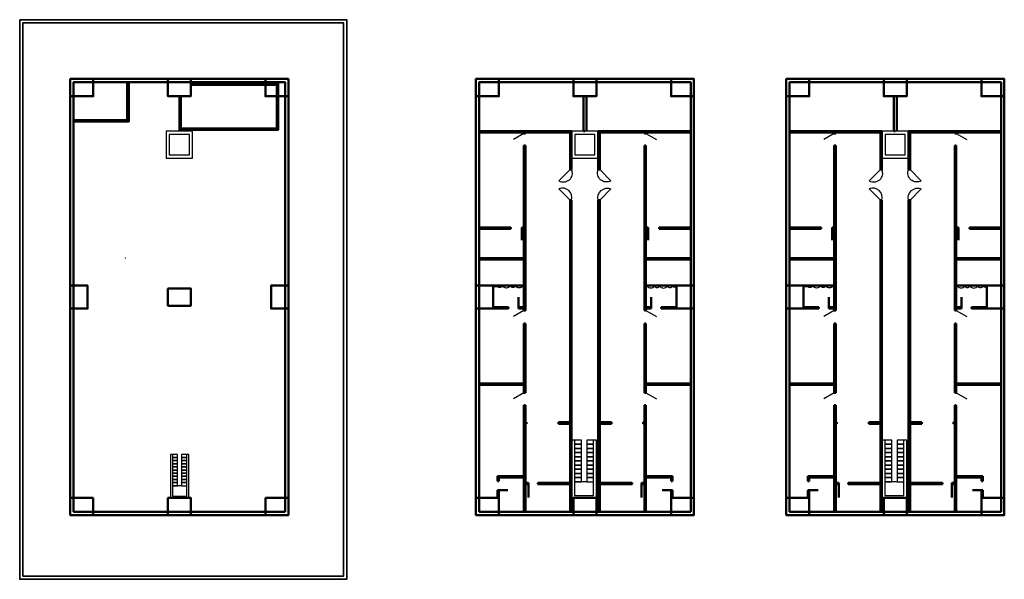
# Model space of a CAD drawing. Units: feet. Extents: x 1080 to 13444, y 870 to 7060.
# Tile 1 of 5: x 1080 to 3789, y 870 to 2410. Entities that reach past the tile are written whole.
import ezdxf

# ---------------------------------------------------------------- set-up
doc = ezdxf.new("R2010")
doc.units = ezdxf.units.FT
for name, color, linetype, lineweight in [('A-ANNO-NPLT', 8, 'Continuous', 13), ('A-COLS', 1, 'Continuous', 50), ('A-DOOR', 4, 'Continuous', 25), ('A-FLOR-EVTR', 6, 'Continuous', 25), ('A-FLOR-STRS', 2, 'Continuous', 25), ('A-GLAZ', 3, 'Continuous', 25), ('A-WALL', 7, 'Continuous', 50), ('C-PROP', 3, 'Continuous', 35)]:
    doc.layers.add(name, color=color, linetype=linetype, lineweight=lineweight)

# ---------------------------------------------------------------- blocks, each defined once
blk = doc.blocks.new('DOOR-SWING-A')
blk.add_line((30.9, 34), (0, 3.5))
blk.add_arc((12.6, 24.3), 24.3, 238.69, 23.7025)
blk = doc.blocks.new('DOOR-SWING-B')
blk.add_line((0, 30.5), (30.9, 0))
blk.add_arc((10.2, 7), 25.6, 344.0766, 113.531)

msp = doc.modelspace()

# ---------------------------------------------------------------- linework, layer by layer
at = {"layer": 'A-ANNO-NPLT'}
for p in [(1370.9, 1754.2), (2471.5, 1405), (2799.2, 1405), (3325.4, 1405), (3653.1, 1405)]:
    msp.add_point(p, dxfattribs=at)
at = {"layer": 'A-COLS'}
for points in [[(1219.3, 2246.8), (1282.3, 2246.8), (1282.3, 2199.1), (1219.3, 2199.1)], [(1487.8, 2246.8), (1550.8, 2246.8), (1550.8, 2199.1), (1487.8, 2199.1)], [(1756.3, 2246.8), (1819.3, 2246.8), (1819.3, 2199.1), (1756.3, 2199.1)], [(2335.3, 2246.8), (2398.4, 2246.8), (2398.4, 2199.1), (2335.3, 2199.1)], [(2603.8, 2246.8), (2666.8, 2246.8), (2666.8, 2199.1), (2603.8, 2199.1)], [(2872.3, 2246.8), (2935.3, 2246.8), (2935.3, 2199.1), (2872.3, 2199.1)], [(3189.2, 2246.8), (3252.3, 2246.8), (3252.3, 2199.1), (3189.2, 2199.1)], [(3457.7, 2246.8), (3520.7, 2246.8), (3520.7, 2199.1), (3457.7, 2199.1)], [(3726.2, 2246.8), (3789.2, 2246.8), (3789.2, 2199.1), (3726.2, 2199.1)], [(1219.3, 1615.2), (1219.3, 1678.3), (1266.9, 1678.3), (1266.9, 1615.2)], [(1487.8, 1670.6), (1550.8, 1670.6), (1550.8, 1622.9), (1487.8, 1622.9)], [(1819.3, 1678.3), (1819.3, 1615.2), (1771.6, 1615.2), (1771.6, 1678.3)], [(2335.3, 1615.2), (2335.3, 1678.3), (2383, 1678.3), (2383, 1615.2)], [(2935.3, 1678.3), (2935.3, 1615.2), (2887.7, 1615.2), (2887.7, 1678.3)], [(3189.2, 1615.2), (3189.2, 1678.3), (3236.9, 1678.3), (3236.9, 1615.2)], [(3789.2, 1678.3), (3789.2, 1615.2), (3741.6, 1615.2), (3741.6, 1678.3)], [(1282.3, 1094.4), (1219.3, 1094.4), (1219.3, 1046.8), (1282.3, 1046.8)], [(1487.8, 1094.4), (1550.8, 1094.4), (1550.8, 1046.8), (1487.8, 1046.8)], [(1756.3, 1094.4), (1819.3, 1094.4), (1819.3, 1046.8), (1756.3, 1046.8)], [(2398.4, 1094.4), (2335.3, 1094.4), (2335.3, 1046.8), (2398.4, 1046.8)], [(2666.8, 1046.8), (2603.8, 1046.8), (2603.8, 1094.4), (2666.8, 1094.4)], [(2872.3, 1094.4), (2935.3, 1094.4), (2935.3, 1046.8), (2872.3, 1046.8)], [(3252.3, 1094.4), (3189.2, 1094.4), (3189.2, 1046.8), (3252.3, 1046.8)], [(3520.7, 1046.8), (3457.7, 1046.8), (3457.7, 1094.4), (3520.7, 1094.4)], [(3726.2, 1094.4), (3789.2, 1094.4), (3789.2, 1046.8), (3726.2, 1046.8)]]:
    msp.add_lwpolyline(points, close=True, dxfattribs=at)
at = {"layer": 'A-DOOR'}
for p, q in [((2467.5, 2096.8), (2438.6, 2080.5)), ((2803.2, 2096.8), (2832.1, 2080.5)), ((3321.4, 2096.8), (3292.5, 2080.5)), ((3657.1, 2096.8), (3686, 2080.5)), ((2467.5, 1609.3), (2438.6, 1593)), ((2803.2, 1609.3), (2832.1, 1593)), ((3321.4, 1609.3), (3292.5, 1593)), ((3657.1, 1609.3), (3686, 1593)), ((2467.5, 1382.8), (2438.6, 1366.5)), ((2803.2, 1382.8), (2832.1, 1366.5)), ((3321.4, 1382.8), (3292.5, 1366.5)), ((3657.1, 1382.8), (3686, 1366.5))]:
    msp.add_line(p, q, dxfattribs=at)
at = {"layer": 'A-FLOR-EVTR'}
for points in [[(1482.6, 2028.8), (1555.9, 2028.8), (1555.9, 2103.4), (1482.6, 2103.4), (1482.6, 2101.1)], [(1491.7, 2037.8), (1546.8, 2037.8), (1546.8, 2094.3), (1491.7, 2094.3)], [(2598.7, 2028.8), (2672, 2028.8), (2672, 2103.4), (2598.7, 2103.4), (2598.7, 2101.1)], [(2607.8, 2037.8), (2662.9, 2037.8), (2662.9, 2094.3), (2607.8, 2094.3)], [(3452.6, 2028.8), (3525.9, 2028.8), (3525.9, 2103.4), (3452.6, 2103.4), (3452.6, 2101.1)], [(3461.7, 2037.8), (3516.8, 2037.8), (3516.8, 2094.3), (3461.7, 2094.3)]]:
    msp.add_lwpolyline(points, close=True, dxfattribs=at)
at = {"layer": 'A-FLOR-STRS'}
for points in [[(2606.3, 1253.3), (2598.7, 1253.3), (2598.7, 1094.5), (2666.8, 1094.5), (2666.8, 1253.3), (2659.2, 1253.3)], [(3460.2, 1253.3), (3452.6, 1253.3), (3452.6, 1094.5), (3520.7, 1094.5), (3520.7, 1253.3), (3513.1, 1253.3)], [(1500.2, 1213.8), (1494.5, 1213.8), (1494.5, 1094.4), (1545.8, 1094.4), (1545.8, 1213.8), (1540, 1213.8)], [(2640.1, 1138.6), (2606.3, 1138.6), (2606.3, 1100.7), (2659.2, 1100.7), (2659.2, 1138.6)], [(3494, 1138.6), (3460.2, 1138.6), (3460.2, 1100.7), (3513.1, 1100.7), (3513.1, 1138.6)], [(1525.6, 1127.5), (1500.2, 1127.5), (1500.2, 1099), (1540, 1099), (1540, 1127.5)]]:
    msp.add_lwpolyline(points, dxfattribs=at)
for points in [[(2606.3, 1253.3), (2606.3, 1241.8), (2625.4, 1241.8), (2625.4, 1253.3)], [(2640.1, 1253.3), (2640.1, 1241.8), (2659.2, 1241.8), (2659.2, 1253.3)], [(3460.2, 1253.3), (3460.2, 1241.8), (3479.3, 1241.8), (3479.3, 1253.3)], [(3494, 1253.3), (3494, 1241.8), (3513.1, 1241.8), (3513.1, 1253.3)], [(2606.3, 1241.8), (2606.3, 1230.3), (2625.4, 1230.3), (2625.4, 1241.8)], [(2606.3, 1230.3), (2606.3, 1218.9), (2625.4, 1218.9), (2625.4, 1230.3)], [(2640.1, 1241.8), (2640.1, 1230.3), (2659.2, 1230.3), (2659.2, 1241.8)], [(2640.1, 1230.3), (2640.1, 1218.9), (2659.2, 1218.9), (2659.2, 1230.3)], [(3460.2, 1241.8), (3460.2, 1230.3), (3479.3, 1230.3), (3479.3, 1241.8)], [(3460.2, 1230.3), (3460.2, 1218.9), (3479.3, 1218.9), (3479.3, 1230.3)], [(3494, 1241.8), (3494, 1230.3), (3513.1, 1230.3), (3513.1, 1241.8)], [(3494, 1230.3), (3494, 1218.9), (3513.1, 1218.9), (3513.1, 1230.3)], [(1500.2, 1213.8), (1500.2, 1205.2), (1514.6, 1205.2), (1514.6, 1213.8)], [(1500.2, 1205.2), (1500.2, 1196.6), (1514.6, 1196.6), (1514.6, 1205.2)], [(1500.2, 1196.6), (1500.2, 1187.9), (1514.6, 1187.9), (1514.6, 1196.6)], [(1525.6, 1213.8), (1525.6, 1205.2), (1540, 1205.2), (1540, 1213.8)], [(1525.6, 1205.2), (1525.6, 1196.6), (1540, 1196.6), (1540, 1205.2)], [(1525.6, 1196.6), (1525.6, 1187.9), (1540, 1187.9), (1540, 1196.6)], [(2606.3, 1218.9), (2606.3, 1207.4), (2625.4, 1207.4), (2625.4, 1218.9)], [(2606.3, 1207.4), (2606.3, 1195.9), (2625.4, 1195.9), (2625.4, 1207.4)], [(2606.3, 1195.9), (2606.3, 1184.5), (2625.4, 1184.5), (2625.4, 1195.9)], [(2640.1, 1218.9), (2640.1, 1207.4), (2659.2, 1207.4), (2659.2, 1218.9)], [(2640.1, 1207.4), (2640.1, 1195.9), (2659.2, 1195.9), (2659.2, 1207.4)], [(2640.1, 1195.9), (2640.1, 1184.5), (2659.2, 1184.5), (2659.2, 1195.9)], [(3460.2, 1218.9), (3460.2, 1207.4), (3479.3, 1207.4), (3479.3, 1218.9)], [(3460.2, 1207.4), (3460.2, 1195.9), (3479.3, 1195.9), (3479.3, 1207.4)], [(3460.2, 1195.9), (3460.2, 1184.5), (3479.3, 1184.5), (3479.3, 1195.9)], [(3494, 1218.9), (3494, 1207.4), (3513.1, 1207.4), (3513.1, 1218.9)], [(3494, 1207.4), (3494, 1195.9), (3513.1, 1195.9), (3513.1, 1207.4)], [(3494, 1195.9), (3494, 1184.5), (3513.1, 1184.5), (3513.1, 1195.9)], [(1500.2, 1187.9), (1500.2, 1179.3), (1514.6, 1179.3), (1514.6, 1187.9)], [(1500.2, 1179.3), (1500.2, 1170.7), (1514.6, 1170.7), (1514.6, 1179.3)], [(1500.2, 1170.7), (1500.2, 1162.1), (1514.6, 1162.1), (1514.6, 1170.7)], [(1525.6, 1187.9), (1525.6, 1179.3), (1540, 1179.3), (1540, 1187.9)], [(1525.6, 1179.3), (1525.6, 1170.7), (1540, 1170.7), (1540, 1179.3)], [(1525.6, 1170.7), (1525.6, 1162.1), (1540, 1162.1), (1540, 1170.7)], [(2606.3, 1184.5), (2606.3, 1173), (2625.4, 1173), (2625.4, 1184.5)], [(2606.3, 1173), (2606.3, 1161.5), (2625.4, 1161.5), (2625.4, 1173)], [(2640.1, 1184.5), (2640.1, 1173), (2659.2, 1173), (2659.2, 1184.5)], [(2640.1, 1173), (2640.1, 1161.5), (2659.2, 1161.5), (2659.2, 1173)], [(3460.2, 1184.5), (3460.2, 1173), (3479.3, 1173), (3479.3, 1184.5)], [(3460.2, 1173), (3460.2, 1161.5), (3479.3, 1161.5), (3479.3, 1173)], [(3494, 1184.5), (3494, 1173), (3513.1, 1173), (3513.1, 1184.5)], [(3494, 1173), (3494, 1161.5), (3513.1, 1161.5), (3513.1, 1173)], [(1500.2, 1162.1), (1500.2, 1153.4), (1514.6, 1153.4), (1514.6, 1162.1)], [(1500.2, 1153.4), (1500.2, 1144.8), (1514.6, 1144.8), (1514.6, 1153.4)], [(1500.2, 1144.8), (1500.2, 1136.2), (1514.6, 1136.2), (1514.6, 1144.8)], [(1525.6, 1162.1), (1525.6, 1153.4), (1540, 1153.4), (1540, 1162.1)], [(1525.6, 1153.4), (1525.6, 1144.8), (1540, 1144.8), (1540, 1153.4)], [(1525.6, 1144.8), (1525.6, 1136.2), (1540, 1136.2), (1540, 1144.8)], [(2606.3, 1161.5), (2606.3, 1150.1), (2625.4, 1150.1), (2625.4, 1161.5)], [(2606.3, 1150.1), (2606.3, 1138.6), (2625.4, 1138.6), (2625.4, 1150.1)], [(2640.1, 1161.5), (2640.1, 1150.1), (2659.2, 1150.1), (2659.2, 1161.5)], [(2640.1, 1150.1), (2640.1, 1138.6), (2659.2, 1138.6), (2659.2, 1150.1)], [(3460.2, 1161.5), (3460.2, 1150.1), (3479.3, 1150.1), (3479.3, 1161.5)], [(3460.2, 1150.1), (3460.2, 1138.6), (3479.3, 1138.6), (3479.3, 1150.1)], [(3494, 1161.5), (3494, 1150.1), (3513.1, 1150.1), (3513.1, 1161.5)], [(3494, 1150.1), (3494, 1138.6), (3513.1, 1138.6), (3513.1, 1150.1)], [(1500.2, 1136.2), (1500.2, 1127.5), (1514.6, 1127.5), (1514.6, 1136.2)], [(1525.6, 1136.2), (1525.6, 1127.5), (1540, 1127.5), (1540, 1136.2)]]:
    msp.add_lwpolyline(points, close=True, dxfattribs=at)
at = {"layer": 'A-GLAZ'}
for points in [[(2467.2, 1678.3, -0.136738), (2464.2, 1676.9, -0.520567), (2444.2, 1676.9, -0.520567), (2429.9, 1676.9, -0.520567), (2408.4, 1676.9, -0.520567), (2393.5, 1676.9, -0.520567), (2384.5, 1676.9, -0.053369), (2383, 1678.3, -0.053369)], [(2803.5, 1678.3, 0.136738), (2806.5, 1676.9, 0.520567), (2826.5, 1676.9, 0.520567), (2840.7, 1676.9, 0.520567), (2862.3, 1676.9, 0.520567), (2877.2, 1676.9, 0.520567), (2886.1, 1676.9, 0.053369), (2887.7, 1678.3, 0.053369)], [(3321.1, 1678.3, -0.136738), (3318.1, 1676.9, -0.520567), (3298.1, 1676.9, -0.520567), (3283.8, 1676.9, -0.520567), (3262.3, 1676.9, -0.520567), (3247.4, 1676.9, -0.520567), (3238.4, 1676.9, -0.053369), (3236.9, 1678.3, -0.053369)], [(3657.4, 1678.3, 0.136738), (3660.4, 1676.9, 0.520567), (3680.4, 1676.9, 0.520567), (3694.6, 1676.9, 0.520567), (3716.2, 1676.9, 0.520567), (3731.1, 1676.9, 0.520567), (3740, 1676.9, 0.053369), (3741.6, 1678.3, 0.053369)]]:
    msp.add_lwpolyline(points, format="xyb", dxfattribs=at)
at = {"layer": 'A-WALL'}
for p, q in [((2631.3, 2103.4), (2631.3, 2199.1)), ((2639.3, 2103.4), (2639.3, 2199.1)), ((3485.2, 2103.4), (3485.2, 2199.1)), ((3493.2, 2103.4), (3493.2, 2199.1)), ((2598.7, 2103.4), (2344.3, 2103.4)), ((2598.7, 2099.4), (2344.3, 2099.4)), ((2467.5, 2103.4), (2467.5, 2096.8)), ((2471.5, 2096.8), (2467.5, 2096.8)), ((2471.5, 2103.4), (2471.5, 2096.8)), ((2594.7, 2103.4), (2594.7, 1997.4)), ((2598.7, 2103.4), (2598.7, 1997.4)), ((2635.3, 2103.4), (2631.3, 2103.4)), ((2672, 2103.4), (2926.3, 2103.4)), ((2672, 2103.4), (2672, 1997.4)), ((2672, 2099.4), (2926.3, 2099.4)), ((2676, 2103.4), (2676, 1997.4)), ((2799.2, 2103.4), (2799.2, 2096.8)), ((2799.2, 2096.8), (2803.2, 2096.8)), ((2803.2, 2103.4), (2803.2, 2096.8)), ((3452.6, 2103.4), (3198.2, 2103.4)), ((3452.6, 2099.4), (3198.2, 2099.4)), ((3321.4, 2103.4), (3321.4, 2096.8)), ((3325.4, 2096.8), (3321.4, 2096.8)), ((3325.4, 2103.4), (3325.4, 2096.8)), ((3448.6, 2103.4), (3448.6, 1997.4)), ((3452.6, 2103.4), (3452.6, 1997.4)), ((3489.2, 2103.4), (3485.2, 2103.4)), ((3525.9, 2103.4), (3780.2, 2103.4)), ((3525.9, 2103.4), (3525.9, 1997.4)), ((3525.9, 2099.4), (3780.2, 2099.4)), ((3529.9, 2103.4), (3529.9, 1997.4)), ((3653.1, 2103.4), (3653.1, 2096.8)), ((3653.1, 2096.8), (3657.1, 2096.8)), ((3657.1, 2103.4), (3657.1, 2096.8)), ((2467.5, 2064.1), (2471.5, 2064.1)), ((2467.5, 2064.1), (2467.5, 1609.3)), ((2471.5, 2064.1), (2471.5, 1609.3)), ((2799.2, 2064.1), (2799.2, 1609.3)), ((2803.2, 2064.1), (2799.2, 2064.1)), ((2803.2, 2064.1), (2803.2, 1609.3)), ((3321.4, 2064.1), (3321.4, 1609.3)), ((3321.4, 2064.1), (3325.4, 2064.1)), ((3325.4, 2064.1), (3325.4, 1609.3)), ((3653.1, 2064.1), (3653.1, 1609.3)), ((3657.1, 2064.1), (3653.1, 2064.1)), ((3657.1, 2064.1), (3657.1, 1609.3)), ((2594.7, 1997.4), (2598.7, 1997.4)), ((2672, 1997.4), (2676, 1997.4)), ((3448.6, 1997.4), (3452.6, 1997.4)), ((3525.9, 1997.4), (3529.9, 1997.4)), ((2598.7, 1913.7), (2594.7, 1913.7)), ((2594.7, 1913.7), (2594.7, 1302.3)), ((2598.7, 1913.7), (2598.7, 1302.3)), ((2672, 1913.7), (2672, 1302.3)), ((2672, 1913.7), (2676, 1913.7)), ((2676, 1913.7), (2676, 1302.3)), ((3448.6, 1913.7), (3448.6, 1302.3)), ((3452.6, 1913.7), (3448.6, 1913.7)), ((3452.6, 1913.7), (3452.6, 1302.3)), ((3525.9, 1913.7), (3525.9, 1302.3)), ((3525.9, 1913.7), (3529.9, 1913.7)), ((3529.9, 1913.7), (3529.9, 1302.3)), ((2344.3, 1754.2), (2344.3, 1838.4)), ((2344.3, 1838.4), (2431.3, 1838.4)), ((2344.3, 1834.4), (2431.3, 1834.4)), ((2431.3, 1838.4), (2431.3, 1834.4)), ((2461.3, 1834.4), (2461.3, 1838.4)), ((2461.3, 1838.4), (2467.5, 1838.4)), ((2461.3, 1834.4), (2467.5, 1834.4)), ((2461.3, 1834.4), (2461.3, 1803.5)), ((2809.4, 1838.4), (2803.2, 1838.4)), ((2809.4, 1834.4), (2803.2, 1834.4)), ((2809.4, 1834.4), (2809.4, 1838.4)), ((2809.4, 1834.4), (2809.4, 1803.5)), ((2926.3, 1838.4), (2839.3, 1838.4)), ((2839.3, 1838.4), (2839.3, 1834.4)), ((2926.3, 1834.4), (2839.3, 1834.4)), ((3198.2, 1754.2), (3198.2, 1838.4)), ((3198.2, 1838.4), (3285.2, 1838.4)), ((3198.2, 1834.4), (3285.2, 1834.4)), ((3285.2, 1838.4), (3285.2, 1834.4)), ((3315.2, 1838.4), (3321.4, 1838.4)), ((3315.2, 1834.4), (3315.2, 1838.4)), ((3315.2, 1834.4), (3321.4, 1834.4)), ((3315.2, 1834.4), (3315.2, 1803.5)), ((3663.3, 1838.4), (3657.1, 1838.4)), ((3663.3, 1834.4), (3657.1, 1834.4)), ((3663.3, 1834.4), (3663.3, 1838.4)), ((3663.3, 1834.4), (3663.3, 1803.5)), ((3780.2, 1838.4), (3693.2, 1838.4)), ((3693.2, 1838.4), (3693.2, 1834.4)), ((3780.2, 1834.4), (3693.2, 1834.4)), ((2471.5, 1754.2), (2344.3, 1754.2)), ((2471.5, 1750.2), (2344.3, 1750.2)), ((2799.2, 1754.2), (2926.3, 1754.2)), ((2799.2, 1750.2), (2926.3, 1750.2)), ((3325.4, 1754.2), (3198.2, 1754.2)), ((3325.4, 1750.2), (3198.2, 1750.2)), ((3653.1, 1754.2), (3780.2, 1754.2)), ((3653.1, 1750.2), (3780.2, 1750.2)), ((2383, 1678.3), (2467.5, 1678.3)), ((2887.7, 1678.3), (2803.2, 1678.3)), ((3236.9, 1678.3), (3321.4, 1678.3)), ((3741.6, 1678.3), (3657.1, 1678.3)), ((2452.7, 1619.2), (2452.7, 1646)), ((2817.9, 1619.2), (2817.9, 1646)), ((3306.6, 1619.2), (3306.6, 1646)), ((3671.8, 1619.2), (3671.8, 1646)), ((2383, 1619.2), (2425.2, 1619.2)), ((2383, 1615.2), (2425.2, 1615.2)), ((2425.2, 1619.2), (2425.2, 1615.2)), ((2452.7, 1615.2), (2452.7, 1619.2)), ((2452.7, 1619.2), (2467.5, 1619.2)), ((2452.7, 1615.2), (2467.5, 1615.2)), ((2471.5, 1609.3), (2467.5, 1609.3)), ((2799.2, 1609.3), (2803.2, 1609.3)), ((2817.9, 1619.2), (2803.2, 1619.2)), ((2817.9, 1615.2), (2803.2, 1615.2)), ((2817.9, 1615.2), (2817.9, 1619.2)), ((2887.7, 1619.2), (2845.4, 1619.2)), ((2845.4, 1619.2), (2845.4, 1615.2)), ((2887.7, 1615.2), (2845.4, 1615.2)), ((3236.9, 1619.2), (3279.1, 1619.2)), ((3236.9, 1615.2), (3279.1, 1615.2)), ((3279.1, 1619.2), (3279.1, 1615.2)), ((3306.6, 1619.2), (3321.4, 1619.2)), ((3306.6, 1615.2), (3306.6, 1619.2)), ((3306.6, 1615.2), (3321.4, 1615.2)), ((3325.4, 1609.3), (3321.4, 1609.3)), ((3653.1, 1609.3), (3657.1, 1609.3)), ((3671.8, 1619.2), (3657.1, 1619.2)), ((3671.8, 1615.2), (3657.1, 1615.2)), ((3671.8, 1615.2), (3671.8, 1619.2)), ((3741.6, 1619.2), (3699.3, 1619.2)), ((3699.3, 1619.2), (3699.3, 1615.2)), ((3741.6, 1615.2), (3699.3, 1615.2)), ((2467.5, 1573.7), (2471.5, 1573.7)), ((2467.5, 1573.7), (2467.5, 1382.8)), ((2471.5, 1573.7), (2471.5, 1382.8)), ((2799.2, 1573.7), (2799.2, 1382.8)), ((2803.2, 1573.7), (2799.2, 1573.7)), ((2803.2, 1573.7), (2803.2, 1382.8)), ((3321.4, 1573.7), (3321.4, 1382.8)), ((3321.4, 1573.7), (3325.4, 1573.7)), ((3325.4, 1573.7), (3325.4, 1382.8)), ((3653.1, 1573.7), (3653.1, 1382.8)), ((3657.1, 1573.7), (3653.1, 1573.7)), ((3657.1, 1573.7), (3657.1, 1382.8)), ((2471.5, 1409), (2344.3, 1409)), ((2799.2, 1409), (2926.3, 1409)), ((3325.4, 1409), (3198.2, 1409)), ((3653.1, 1409), (3780.2, 1409)), ((2471.5, 1405), (2344.3, 1405)), ((2467.5, 1382.8), (2471.5, 1382.8)), ((2799.2, 1405), (2926.3, 1405)), ((2803.2, 1382.8), (2799.2, 1382.8)), ((3325.4, 1405), (3198.2, 1405)), ((3321.4, 1382.8), (3325.4, 1382.8)), ((3653.1, 1405), (3780.2, 1405)), ((3657.1, 1382.8), (3653.1, 1382.8)), ((2471.5, 1348.9), (2467.5, 1348.9)), ((2467.5, 1348.9), (2467.5, 1302.3)), ((2471.5, 1348.9), (2471.5, 1302.3)), ((2799.2, 1348.9), (2799.2, 1302.3)), ((2799.2, 1348.9), (2803.2, 1348.9)), ((2803.2, 1348.9), (2803.2, 1302.3)), ((3321.4, 1348.9), (3321.4, 1302.3)), ((3325.4, 1348.9), (3321.4, 1348.9)), ((3325.4, 1348.9), (3325.4, 1302.3)), ((3653.1, 1348.9), (3653.1, 1302.3)), ((3653.1, 1348.9), (3657.1, 1348.9)), ((3657.1, 1348.9), (3657.1, 1302.3)), ((2467.5, 1302.3), (2474.7, 1302.3)), ((2467.5, 1055.8), (2467.5, 1302.3)), ((2471.5, 1055.8), (2471.5, 1302.3)), ((2474.7, 1298.3), (2474.7, 1302.3)), ((2562.2, 1302.3), (2562.2, 1298.3)), ((2562.2, 1302.3), (2598.7, 1302.3)), ((2594.7, 1302.3), (2594.7, 1131.4)), ((2598.7, 1302.3), (2598.7, 1131.4)), ((2708.5, 1302.3), (2672, 1302.3)), ((2672, 1302.3), (2672, 1131.4)), ((2676, 1302.3), (2676, 1131.4)), ((2708.5, 1302.3), (2708.5, 1298.3)), ((2803.2, 1302.3), (2795.9, 1302.3)), ((2795.9, 1298.3), (2795.9, 1302.3)), ((2799.2, 1055.8), (2799.2, 1302.3)), ((2803.2, 1055.8), (2803.2, 1302.3)), ((3321.4, 1055.8), (3321.4, 1302.3)), ((3321.4, 1302.3), (3328.6, 1302.3)), ((3325.4, 1055.8), (3325.4, 1302.3)), ((3328.6, 1298.3), (3328.6, 1302.3)), ((3416.1, 1302.3), (3452.6, 1302.3)), ((3416.1, 1302.3), (3416.1, 1298.3)), ((3448.6, 1302.3), (3448.6, 1131.4)), ((3452.6, 1302.3), (3452.6, 1131.4)), ((3562.4, 1302.3), (3525.9, 1302.3)), ((3525.9, 1302.3), (3525.9, 1131.4)), ((3529.9, 1302.3), (3529.9, 1131.4)), ((3562.4, 1302.3), (3562.4, 1298.3)), ((3657.1, 1302.3), (3649.8, 1302.3)), ((3649.8, 1298.3), (3649.8, 1302.3)), ((3653.1, 1055.8), (3653.1, 1302.3)), ((3657.1, 1055.8), (3657.1, 1302.3)), ((2471.5, 1298.3), (2474.7, 1298.3)), ((2562.2, 1298.3), (2598.7, 1298.3)), ((2708.5, 1298.3), (2672, 1298.3)), ((2799.2, 1298.3), (2795.9, 1298.3)), ((3325.4, 1298.3), (3328.6, 1298.3)), ((3416.1, 1298.3), (3452.6, 1298.3)), ((3562.4, 1298.3), (3525.9, 1298.3)), ((3653.1, 1298.3), (3649.8, 1298.3)), ((2394.4, 1154.2), (2467.5, 1154.2)), ((2394.4, 1140.1), (2394.4, 1154.2)), ((2398.4, 1140.1), (2394.4, 1140.1)), ((2398.4, 1140.1), (2398.4, 1154.2)), ((2398.4, 1150.2), (2467.5, 1150.2)), ((2876.3, 1154.2), (2803.2, 1154.2)), ((2872.3, 1150.2), (2803.2, 1150.2)), ((2872.3, 1140.1), (2872.3, 1154.2)), ((2872.3, 1140.1), (2876.3, 1140.1)), ((2876.3, 1140.1), (2876.3, 1154.2)), ((3248.3, 1140.1), (3248.3, 1154.2)), ((3248.3, 1154.2), (3321.4, 1154.2)), ((3252.3, 1140.1), (3248.3, 1140.1)), ((3252.3, 1140.1), (3252.3, 1154.2)), ((3252.3, 1150.2), (3321.4, 1150.2)), ((3730.2, 1154.2), (3657.1, 1154.2)), ((3726.2, 1150.2), (3657.1, 1150.2)), ((3726.2, 1140.1), (3726.2, 1154.2)), ((3726.2, 1140.1), (3730.2, 1140.1)), ((3730.2, 1140.1), (3730.2, 1154.2)), ((2394.4, 1094.4), (2394.4, 1115)), ((2394.4, 1115), (2398.4, 1115)), ((2398.4, 1094.4), (2398.4, 1115)), ((2398.4, 1115), (2422.9, 1115)), ((2479.9, 1135.4), (2471.5, 1135.4)), ((2479.9, 1131.4), (2471.5, 1131.4)), ((2479.9, 1135.4), (2479.9, 1131.4)), ((2479.9, 1131.4), (2479.9, 1094.7)), ((2598.7, 1135.4), (2505.5, 1135.4)), ((2505.5, 1131.4), (2505.5, 1135.4)), ((2598.7, 1131.4), (2505.5, 1131.4)), ((2594.7, 1131.4), (2594.7, 1055.8)), ((2598.7, 1131.4), (2598.7, 1055.8)), ((2672, 1135.4), (2765.2, 1135.4)), ((2672, 1131.4), (2765.2, 1131.4)), ((2672, 1131.4), (2672, 1055.8)), ((2676, 1131.4), (2676, 1055.8)), ((2765.2, 1131.4), (2765.2, 1135.4)), ((2790.7, 1135.4), (2799.2, 1135.4)), ((2790.7, 1135.4), (2790.7, 1131.4)), ((2790.7, 1131.4), (2799.2, 1131.4)), ((2790.7, 1131.4), (2790.7, 1094.7)), ((2872.3, 1115), (2847.8, 1115)), ((2872.3, 1094.4), (2872.3, 1115)), ((2876.3, 1115), (2872.3, 1115)), ((2876.3, 1094.4), (2876.3, 1115)), ((3248.3, 1094.4), (3248.3, 1115)), ((3248.3, 1115), (3252.3, 1115)), ((3252.3, 1094.4), (3252.3, 1115)), ((3252.3, 1115), (3276.8, 1115)), ((3333.8, 1135.4), (3325.4, 1135.4)), ((3333.8, 1131.4), (3325.4, 1131.4)), ((3333.8, 1135.4), (3333.8, 1131.4)), ((3333.8, 1131.4), (3333.8, 1094.7)), ((3452.6, 1135.4), (3359.4, 1135.4)), ((3359.4, 1131.4), (3359.4, 1135.4)), ((3452.6, 1131.4), (3359.4, 1131.4)), ((3448.6, 1131.4), (3448.6, 1055.8)), ((3452.6, 1131.4), (3452.6, 1055.8)), ((3525.9, 1135.4), (3619.1, 1135.4)), ((3525.9, 1131.4), (3619.1, 1131.4)), ((3525.9, 1131.4), (3525.9, 1055.8)), ((3529.9, 1131.4), (3529.9, 1055.8)), ((3619.1, 1131.4), (3619.1, 1135.4)), ((3644.6, 1135.4), (3653.1, 1135.4)), ((3644.6, 1135.4), (3644.6, 1131.4)), ((3644.6, 1131.4), (3653.1, 1131.4)), ((3644.6, 1131.4), (3644.6, 1094.7)), ((3726.2, 1115), (3701.7, 1115)), ((3726.2, 1094.4), (3726.2, 1115)), ((3730.2, 1115), (3726.2, 1115)), ((3730.2, 1094.4), (3730.2, 1115))]:
    msp.add_line(p, q, dxfattribs=at)
for points in [[(1819.3, 1046.8), (1219.3, 1046.8), (1219.3, 2246.8), (1819.3, 2246.8)], [(1810.3, 1055.8), (1228.3, 1055.8), (1228.3, 2237.8), (1810.3, 2237.8)], [(2935.3, 1046.8), (2335.3, 1046.8), (2335.3, 2246.8), (2935.3, 2246.8)], [(2926.3, 1055.8), (2344.3, 1055.8), (2344.3, 2237.8), (2926.3, 2237.8)], [(3789.2, 1046.8), (3189.2, 1046.8), (3189.2, 2246.8), (3789.2, 2246.8)], [(3780.2, 1055.8), (3198.2, 1055.8), (3198.2, 2237.8), (3780.2, 2237.8)]]:
    msp.add_lwpolyline(points, close=True, dxfattribs=at)
for points in [[(1376.1, 2237.8), (1376.1, 2133.4), (1228.3, 2133.4)], [(1380.1, 2237.8), (1380.1, 2129.4), (1228.3, 2129.4)], [(1550.8, 2234.6), (1667.1, 2234.6), (1791.1, 2234.6), (1791.1, 2106.6), (1547.1, 2106.6), (1519.3, 2106.6), (1519.3, 2199.1)], [(1550.8, 2230.6), (1667.1, 2230.6), (1787.1, 2230.6), (1787.1, 2110.6), (1547.1, 2110.6), (1523.3, 2110.6), (1523.3, 2199.1)]]:
    msp.add_lwpolyline(points, dxfattribs=at)
at = {"layer": 'C-PROP'}
for points in [[(1080, 2410), (1980, 2410), (1980, 870), (1080, 870)], [(1089, 2401), (1971, 2401), (1971, 879), (1089, 879)]]:
    msp.add_lwpolyline(points, close=True, dxfattribs=at)

# ---------------------------------------------------------------- block references
at = {"layer": 'A-DOOR'}
for name, p in [('DOOR-SWING-A', (2563.8, 1963.4)), ('DOOR-SWING-A', (3417.7, 1963.4)), ('DOOR-SWING-B', (2563.8, 1913.7)), ('DOOR-SWING-B', (3417.7, 1913.7))]:
    msp.add_blockref(name, p, dxfattribs=at)
at = {"layer": 'A-DOOR', "extrusion": (0, 0, -1), "zscale": -1, "rotation": 359.9998145993619}
for name, p in [('DOOR-SWING-A', (-2706.9, 1963.4)), ('DOOR-SWING-A', (-3560.8, 1963.4)), ('DOOR-SWING-B', (-2706.9, 1913.7)), ('DOOR-SWING-B', (-3560.8, 1913.7))]:
    msp.add_blockref(name, p, dxfattribs=at)

doc.saveas('drawing.dxf')
